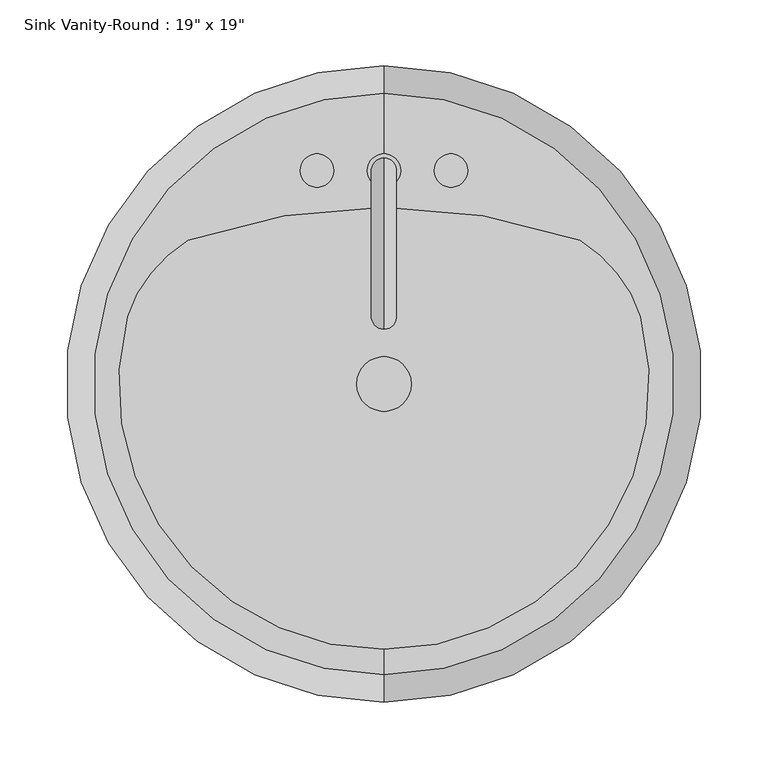
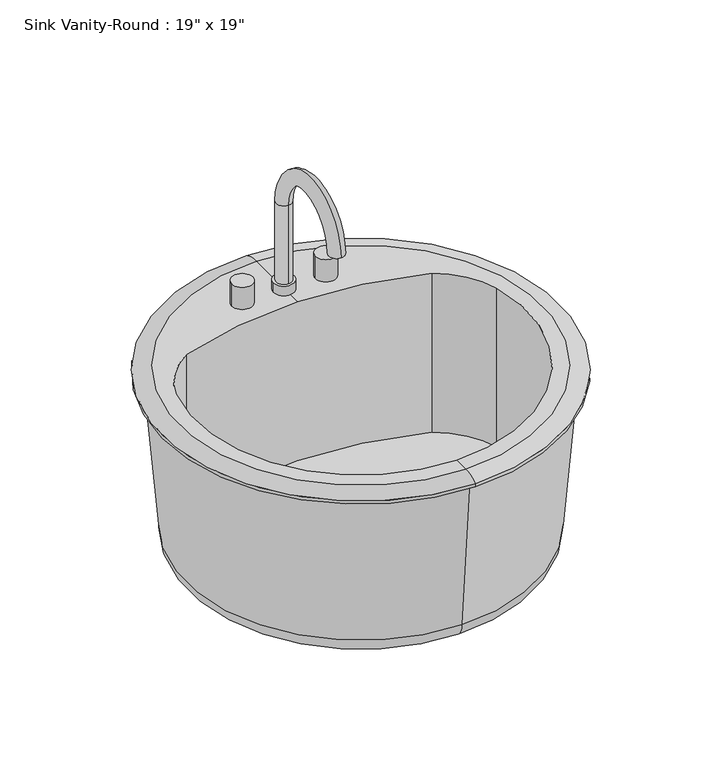
"""IFC4 building model written with IfcOpenShell, lengths in millimetres: flow terminal geometry."""

from ifc_helpers import new_model, si_unit, point, frame, frame_2d, origin, place, context, project, spatial, polyline, circle_curve, ellipse_curve, trimmed, segment, composite_curve, outline, extrude, source, transform, mapped, element, save
from ifc_brep_helpers import plane_surface, cylinder_surface, revolved_surface, advanced_brep


def flow_terminal_d49f872f(model_context):
    return source(origin(), model_context, "Body", "SolidModel", [
        advanced_brep(
        [(83.9517406, 247.0927185, 796.925), (109.3517406, 247.0927185, 796.925), (96.6517406, 237.5677185, 909.6375), (96.6517406, 256.6177185, 909.6375), (96.6517406, 256.6177185, 809.1602909), (96.6517406, 237.5677185, 809.1602909), (96.6517406, 145.7775038, 909.6375), (96.6517406, 126.7275038, 909.6375), (83.9517406, 247.0927185, 809.1602909), (109.3517406, 247.0927185, 809.1602909)],
        [
            (0, 1, circle_curve(frame((96.6517406, 247.0927185, 796.925), z_axis=(0.0, 0.0, -1.0), x_axis=(1.0, 0.0, 0.0)), 12.7)),
            (1, 0, circle_curve(frame((96.6517406, 247.0927185, 796.925), z_axis=(0.0, 0.0, -1.0), x_axis=(1.0, 0.0, 0.0)), 12.7)),
            (2, 3, circle_curve(frame((96.6517406, 247.0927185, 909.6375), z_axis=(0.0, 0.0, -1.0), x_axis=(0.0, 1.0, 0.0)), 9.525)),
            (3, 4),
            (4, 5, circle_curve(frame((96.6517406, 247.0927185, 809.1602909), z_axis=(0.0, 0.0, 1.0), x_axis=(0.0, 1.0, 0.0)), 9.525)),
            (5, 2),
            (3, 2, circle_curve(frame((96.6517406, 247.0927185, 909.6375), z_axis=(0.0, 0.0, -1.0), x_axis=(0.0, 1.0, 0.0)), 9.525)),
            (5, 4, circle_curve(frame((96.6517406, 247.0927185, 809.1602909), z_axis=(0.0, 0.0, 1.0), x_axis=(0.0, 1.0, 0.0)), 9.525)),
            (6, 7, circle_curve(frame((96.6517406, 136.2525038, 909.6375), z_axis=(0.0, 0.0, -1.0), x_axis=(0.0, -1.0, 0.0)), 9.525)),
            (7, 6, circle_curve(frame((96.6517406, 136.2525038, 909.6375), z_axis=(0.0, 0.0, -1.0), x_axis=(0.0, -1.0, 0.0)), 9.525)),
            (2, 6, circle_curve(frame((96.6517406, 191.6726112, 909.6375), z_axis=(1.0, 0.0, 0.0), x_axis=(0.0, 1.0, 0.0)), 45.8951073)),
            (7, 3, circle_curve(frame((96.6517406, 191.6726112, 909.6375), z_axis=(-1.0, 0.0, 0.0), x_axis=(0.0, 1.0, 0.0)), 64.9451073)),
            (8, 9, circle_curve(frame((96.6517406, 247.0927185, 809.1602909), z_axis=(0.0, 0.0, 1.0), x_axis=(1.0, 0.0, 0.0)), 12.7)),
            (9, 8, circle_curve(frame((96.6517406, 247.0927185, 809.1602909), z_axis=(0.0, 0.0, 1.0), x_axis=(1.0, 0.0, 0.0)), 12.7)),
            (8, 0),
            (1, 9),
        ],
        [
            plane_surface(frame((96.6517406, 237.5677185, 796.925), z_axis=(0.0, 0.0, -1.0), x_axis=(1.0, 0.0, 0.0))),
            cylinder_surface(frame((96.6517406, 247.0927185, 796.925), z_axis=(0.0, 0.0, -1.0), x_axis=(0.0, 1.0, 0.0)), 9.525),
            plane_surface(frame((96.6517406, 191.6726112, 909.6375), z_axis=(0.0, 0.0, -1.0), x_axis=(0.0, -1.0, 0.0))),
            revolved_surface(trimmed(ellipse_curve(frame((96.6517406, 247.0927185, 909.6375), z_axis=(0.0, 0.0, -1.0), x_axis=(0.0, 1.0, 0.0)), 9.525, 9.525), [point((96.6517406, 237.5677185, 909.6375))], [point((96.6517406, 256.6177185, 909.6375))], True, "CARTESIAN"), (96.6517406, 191.6726112, 909.6375), (1.0, 0.0, 0.0)),
            revolved_surface(trimmed(ellipse_curve(frame((96.6517406, 247.0927185, 909.6375), z_axis=(0.0, 0.0, -1.0), x_axis=(0.0, 1.0, 0.0)), 9.525, 9.525), [point((96.6517406, 256.6177185, 909.6375))], [point((96.6517406, 237.5677185, 909.6375))], True, "CARTESIAN"), (96.6517406, 191.6726112, 909.6375), (1.0, 0.0, 0.0)),
            plane_surface(frame((109.3517406, 247.0927185, 809.1602909), z_axis=(0.0, 0.0, 1.0), x_axis=(0.0, 1.0, 0.0))),
            cylinder_surface(frame((96.6517406, 247.0927185, 796.925), z_axis=(0.0, 0.0, 1.0), x_axis=(1.0, 0.0, 0.0)), 12.7),
        ],
        [
            (0, [[1, 2]]),
            (1, [[3, 4, 5, 6]]),
            (1, [[7, -6, 8, -4]]),
            (2, [[9, 10]]),
            (3, [[-3, 11, -10, 12]]),
            (4, [[-7, -12, -9, -11]]),
            (5, [[13, 14], [-5, -8]]),
            (6, [[-13, 15, -2, 16]]),
            (6, [[-14, -16, -1, -15]]),
        ],
    ),
        extrude(outline(composite_curve([segment(trimmed(circle_curve(frame_2d((45.8517406, 247.0927185)), 12.7), [point((33.1517406, 247.0927185))], [point((58.5517406, 247.0927185))], False, "CARTESIAN"), True, "CONTINUOUS"), segment(trimmed(circle_curve(frame_2d((45.8517406, 247.0927185)), 12.7), [point((58.5517406, 247.0927185))], [point((33.1517406, 247.0927185))], False, "CARTESIAN"), True, "CONTINUOUS")], self_intersect=False)), frame((0.0, 0.0, 796.925), z_axis=(0.0, 0.0, 1.0), x_axis=(1.0, 0.0, 0.0)), (0.0, 0.0, 1.0), 28.575),
        extrude(outline(composite_curve([segment(trimmed(circle_curve(frame_2d((147.4517406, 247.0927185)), 12.7), [point((134.7517406, 247.0927185))], [point((160.1517406, 247.0927185))], False, "CARTESIAN"), True, "CONTINUOUS"), segment(trimmed(circle_curve(frame_2d((147.4517406, 247.0927185)), 12.7), [point((160.1517406, 247.0927185))], [point((134.7517406, 247.0927185))], False, "CARTESIAN"), True, "CONTINUOUS")], self_intersect=False)), frame((0.0, 0.0, 796.925), z_axis=(0.0, 0.0, 1.0), x_axis=(1.0, 0.0, 0.0)), (0.0, 0.0, 1.0), 28.575),
        extrude(outline(composite_curve([segment(trimmed(circle_curve(frame_2d((96.6517406, 85.1677185)), 20.6375), [point((76.0142406, 85.1677185))], [point((117.2892406, 85.1677185))], False, "CARTESIAN"), True, "CONTINUOUS"), segment(trimmed(circle_curve(frame_2d((96.6517406, 85.1677185)), 20.6375), [point((117.2892406, 85.1677185))], [point((76.0142406, 85.1677185))], False, "CARTESIAN"), True, "CONTINUOUS")], self_intersect=False)), frame((0.0, 0.0, 571.5), z_axis=(0.0, 0.0, 1.0), x_axis=(1.0, 0.0, 0.0)), (0.0, 0.0, 1.0), 21.1842611),
        advanced_brep(
        [(96.6517406, -135.3870093, 796.925), (96.6517406, 305.7224463, 796.925), (96.6517406, 326.4677185, 791.36875), (96.6517406, -156.1322815, 791.36875), (96.6517406, -116.2405705, 796.925), (-98.1703414, 136.2525038, 796.925), (-52.1534933, 194.0861398, 796.925), (96.6517406, 219.2662048, 796.925), (245.4569744, 194.0861398, 796.925), (291.4738225, 136.2525038, 796.925), (96.6517406, -107.1264028, 571.5), (96.6517406, 277.4618398, 571.5), (96.6517406, 85.1677185, 571.5), (96.6517406, -127.6827361, 592.6842611), (96.6517406, 298.0181731, 592.6842611), (96.6517406, -144.2260315, 787.4), (96.6517406, 314.5614685, 787.4), (96.6517406, -156.1322815, 787.4), (96.6517406, 326.4677185, 787.4), (245.4569744, 194.0861398, 592.6842611), (-52.1534933, 194.0861398, 592.6842611), (-98.1703414, 136.2525038, 592.6842611), (291.4738225, 136.2525038, 592.6842611)],
        [
            (0, 1, circle_curve(frame((96.6517406, 85.1677185, 796.925), z_axis=(0.0, 0.0, -1.0), x_axis=(0.0, 1.0, 0.0)), 220.5547278)),
            (1, 2, circle_curve(frame((96.6517406, 309.4374616, 769.289434), z_axis=(-1.0, 0.0, 0.0), x_axis=(0.0, 1.0, 0.0)), 27.8841505)),
            (2, 3, circle_curve(frame((96.6517406, 85.1677185, 791.36875), z_axis=(0.0, 0.0, 1.0), x_axis=(0.0, 1.0, 0.0)), 241.3)),
            (3, 0, circle_curve(frame((96.6517406, -139.1020246, 769.289434), z_axis=(-1.0, 0.0, 0.0), x_axis=(0.0, -1.0, 0.0)), 27.8841505)),
            (1, 0, circle_curve(frame((96.6517406, 85.1677185, 796.925), z_axis=(0.0, 0.0, -1.0), x_axis=(0.0, 1.0, 0.0)), 220.5547278)),
            (3, 2, circle_curve(frame((96.6517406, 85.1677185, 791.36875), z_axis=(0.0, 0.0, 1.0), x_axis=(0.0, 1.0, 0.0)), 241.3)),
            (0, 4),
            (4, 5, circle_curve(frame((96.6517406, 85.1677185, 796.925), z_axis=(0.0, 0.0, -1.0), x_axis=(1.0, 0.0, 0.0)), 201.408289)),
            (5, 6, circle_curve(frame((1.3689689, 104.2755165, 796.925), z_axis=(0.0, 0.0, -1.0), x_axis=(1.0, 0.0, 0.0)), 104.5495194)),
            (6, 7, circle_curve(frame((96.6517406, -233.0168462, 796.925), z_axis=(0.0, 0.0, -1.0), x_axis=(1.0, 0.0, 0.0)), 452.283051)),
            (7, 1),
            (7, 8, circle_curve(frame((96.6517406, -233.0168462, 796.925), z_axis=(0.0, 0.0, -1.0), x_axis=(1.0, 0.0, 0.0)), 452.283051)),
            (8, 9, circle_curve(frame((191.9345122, 104.2755165, 796.925), z_axis=(0.0, 0.0, -1.0), x_axis=(1.0, 0.0, 0.0)), 104.5495194)),
            (9, 4, circle_curve(frame((96.6517406, 85.1677185, 796.925), z_axis=(0.0, 0.0, -1.0), x_axis=(1.0, 0.0, 0.0)), 201.408289)),
            (10, 11, circle_curve(frame((96.6517406, 85.1677185, 571.5), z_axis=(0.0, 0.0, -1.0), x_axis=(0.0, 1.0, 0.0)), 192.2941213)),
            (11, 12),
            (12, 10),
            (11, 10, circle_curve(frame((96.6517406, 85.1677185, 571.5), z_axis=(0.0, 0.0, -1.0), x_axis=(0.0, 1.0, 0.0)), 192.2941213)),
            (10, 13, circle_curve(frame((96.6517406, -107.1264028, 592.0656396), z_axis=(-1.0, 0.0, 0.0), x_axis=(0.0, -1.0, 0.0)), 20.5656396)),
            (13, 14, circle_curve(frame((96.6517406, 85.1677185, 592.6842611), z_axis=(0.0, 0.0, -1.0), x_axis=(0.0, 1.0, 0.0)), 212.8504546)),
            (14, 11, circle_curve(frame((96.6517406, 277.4618398, 592.0656396), z_axis=(-1.0, 0.0, 0.0), x_axis=(0.0, 1.0, 0.0)), 20.5656396)),
            (14, 13, circle_curve(frame((96.6517406, 85.1677185, 592.6842611), z_axis=(0.0, 0.0, -1.0), x_axis=(0.0, 1.0, 0.0)), 212.8504546)),
            (13, 15),
            (15, 16, circle_curve(frame((96.6517406, 85.1677185, 787.4), z_axis=(0.0, 0.0, -1.0), x_axis=(0.0, 1.0, 0.0)), 229.39375)),
            (16, 14),
            (16, 15, circle_curve(frame((96.6517406, 85.1677185, 787.4), z_axis=(0.0, 0.0, -1.0), x_axis=(0.0, 1.0, 0.0)), 229.39375)),
            (15, 17),
            (17, 18, circle_curve(frame((96.6517406, 85.1677185, 787.4), z_axis=(0.0, 0.0, -1.0), x_axis=(0.0, 1.0, 0.0)), 241.3)),
            (18, 16),
            (18, 17, circle_curve(frame((96.6517406, 85.1677185, 787.4), z_axis=(0.0, 0.0, -1.0), x_axis=(0.0, 1.0, 0.0)), 241.3)),
            (2, 18),
            (17, 3),
            (19, 20, circle_curve(frame((96.6517406, -233.0168462, 592.6842611), z_axis=(0.0, 0.0, 1.0), x_axis=(1.0, 0.0, 0.0)), 452.283051)),
            (20, 21, circle_curve(frame((1.3689689, 104.2755165, 592.6842611), z_axis=(0.0, 0.0, 1.0), x_axis=(1.0, 0.0, 0.0)), 104.5495194)),
            (21, 22, circle_curve(frame((96.6517406, 85.1677185, 592.6842611), z_axis=(0.0, 0.0, 1.0), x_axis=(1.0, 0.0, 0.0)), 201.408289)),
            (22, 19, circle_curve(frame((191.9345122, 104.2755165, 592.6842611), z_axis=(0.0, 0.0, 1.0), x_axis=(1.0, 0.0, 0.0)), 104.5495194)),
            (19, 8),
            (6, 20),
            (5, 21),
            (9, 22),
        ],
        [
            revolved_surface(trimmed(ellipse_curve(frame((96.6517406, 309.4374616, 769.289434), z_axis=(1.0, 0.0, 0.0), x_axis=(0.0, 1.0, 0.0)), 27.8841505, 27.8841505), [point((96.6517406, 326.4677185, 791.36875))], [point((96.6517406, 305.7224463, 796.925))], True, "CARTESIAN"), (96.6517406, 85.1677185, 796.925), (0.0, 0.0, 1.0)),
            plane_surface(frame((96.6517406, 85.1677185, 796.925), z_axis=(0.0, 0.0, 1.0), x_axis=(0.0, 1.0, 0.0))),
            plane_surface(frame((96.6517406, 85.1677185, 571.5), z_axis=(0.0, 0.0, -1.0), x_axis=(0.0, 1.0, 0.0))),
            revolved_surface(trimmed(ellipse_curve(frame((96.6517406, 277.4618398, 592.0656396), z_axis=(1.0, 0.0, 0.0), x_axis=(0.0, 1.0, 0.0)), 20.5656396, 20.5656396), [point((96.6517406, 277.4618398, 571.5))], [point((96.6517406, 298.0181731, 592.6842611))], True, "CARTESIAN"), (96.6517406, 85.1677185, 796.925), (0.0, 0.0, 1.0)),
            revolved_surface(polyline([(96.6517406, 298.0181731, 592.6842611), (96.6517406, 314.5614685, 787.4)]), (96.6517406, 85.1677185, 796.925), (0.0, 0.0, 1.0)),
            plane_surface(frame((96.6517406, 85.1677185, 787.4), z_axis=(0.0, 0.0, -1.0), x_axis=(0.0, 1.0, 0.0))),
            cylinder_surface(frame((96.6517406, 85.1677185, 796.925), z_axis=(0.0, 0.0, 1.0), x_axis=(0.0, 1.0, 0.0)), 241.3),
            plane_surface(frame((548.9347916, -233.0168462, 592.6842611), z_axis=(0.0, 0.0, 1.0), x_axis=(0.0, -1.0, 0.0))),
            revolved_surface(polyline([(548.9347916, -233.0168462, 796.925), (548.9347916, -233.0168462, 592.6842611)]), (96.6517406, -233.0168462, 592.6842611), (0.0, 0.0, 1.0)),
            revolved_surface(polyline([(105.91848829999999, 104.2755165, 796.925), (105.91848829999999, 104.2755165, 592.6842611)]), (1.3689689, 104.2755165, 592.6842611), (0.0, 0.0, 1.0)),
            revolved_surface(polyline([(298.0600296, 85.1677185, 796.925), (298.0600296, 85.1677185, 592.6842611)]), (96.6517406, 85.1677185, 592.6842611), (0.0, 0.0, 1.0)),
            revolved_surface(polyline([(296.4840316, 104.2755165, 796.925), (296.4840316, 104.2755165, 592.6842611)]), (191.9345122, 104.2755165, 592.6842611), (0.0, 0.0, 1.0)),
        ],
        [
            (0, [[1, 2, 3, 4]]),
            (0, [[-2, 5, -4, 6]]),
            (1, [[-1, 7, 8, 9, 10, 11]]),
            (1, [[-5, -11, 12, 13, 14, -7]]),
            (2, [[15, 16, 17]]),
            (2, [[-16, 18, -17]]),
            (3, [[-15, 19, 20, 21]]),
            (3, [[-18, -21, 22, -19]]),
            (4, [[-20, 23, 24, 25]]),
            (4, [[-22, -25, 26, -23]]),
            (5, [[-24, 27, 28, 29]]),
            (5, [[-26, -29, 30, -27]]),
            (6, [[-3, 31, -28, 32]]),
            (6, [[-6, -32, -30, -31]]),
            (7, [[33, 34, 35, 36]]),
            (8, [[-33, 37, -12, -10, 38]]),
            (9, [[-34, -38, -9, 39]]),
            (10, [[-35, -39, -8, -14, 40]]),
            (11, [[-36, -40, -13, -37]]),
        ],
    ),
    ])


if __name__ == "__main__":
    model = new_model("IFC4")
    model_context = context("Model", 3, world=origin())
    ifc_project = project(units=[si_unit("LENGTHUNIT", "METRE", prefix="MILLI")], contexts=[model_context])
    site = spatial("IfcSite", under=ifc_project)
    building = spatial("IfcBuilding", under=site)
    placement = place(None, origin())
    flow_terminal_shape = flow_terminal_d49f872f(model_context)
    element("IfcFlowTerminal", 1, ObjectType="Sink Vanity-Round : 19\" x 19\"", at=placement, inside=building, context=model_context, shape_type="MappedRepresentation", body=[
        mapped(flow_terminal_shape, transform((0.0, 0.0, 0.0), x_axis=(1.0, 0.0, 0.0), y_axis=(0.0, 1.0, 0.0), z_axis=(0.0, 0.0, 1.0))),
    ])
    save(model, "model.ifc")

# Revit data of these elements
# Type "Sink Vanity-Round : 19\" x 19\""
#   Assembly Code = "D2010400"
#   Top Of Counter = 2' - 7"
#   Basin Material = Porcelain, Linen
#   Faucet Material = Steel, Polished
# Element 1 (IfcFlowTerminal, "Sink Vanity-Round : 19\" x 19\"")
#   Materials on its faces: "Porcelain, Linen", "Steel, Polished"
# Materials
#   "Porcelain, Linen": class "Ceramic", colour RGB 249 239 230, transparency 0, Description = "Porcelain, linen", Cost = 0
#   "Steel, Polished": class "Metal", colour RGB 57 57 57, transparency 0, Description = "Polished steel", Cost = 0
